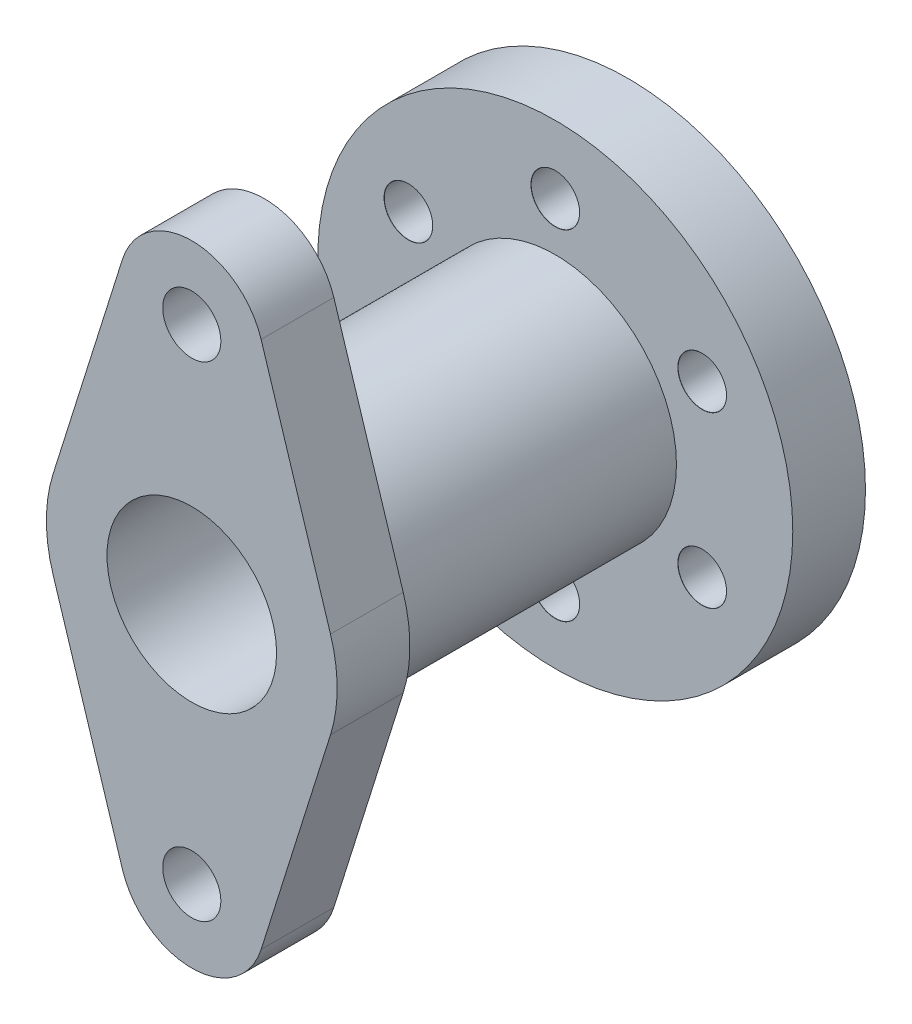
ISO-10303-21;
HEADER;
FILE_DESCRIPTION(('STEP AP214'),'2;1');
FILE_NAME('part.step','',(''),(''),'','','');
FILE_SCHEMA(('AUTOMOTIVE_DESIGN { 1 0 10303 214 1 1 1 1 }'));
ENDSEC;
DATA;
#1=APPLICATION_CONTEXT('core data for automotive mechanical design processes');
#2=APPLICATION_PROTOCOL_DEFINITION('international standard','automotive_design',2000,#1);
#3=PRODUCT_CONTEXT('',#1,'mechanical');
#4=PRODUCT('Part','Part','',(#3));
#5=PRODUCT_RELATED_PRODUCT_CATEGORY('part','',(#4));
#6=PRODUCT_DEFINITION_FORMATION('','',#4);
#7=PRODUCT_DEFINITION_CONTEXT('part definition',#1,'design');
#8=PRODUCT_DEFINITION('design','',#6,#7);
#9=PRODUCT_DEFINITION_SHAPE('','',#8);
#10=(LENGTH_UNIT() NAMED_UNIT(*) SI_UNIT(.MILLI.,.METRE.));
#11=(NAMED_UNIT(*) PLANE_ANGLE_UNIT() SI_UNIT($,.RADIAN.));
#12=(NAMED_UNIT(*) SI_UNIT($,.STERADIAN.) SOLID_ANGLE_UNIT());
#13=UNCERTAINTY_MEASURE_WITH_UNIT(LENGTH_MEASURE(1.E-05),#10,'distance_accuracy_value','');
#14=(GEOMETRIC_REPRESENTATION_CONTEXT(3) GLOBAL_UNCERTAINTY_ASSIGNED_CONTEXT((#13)) GLOBAL_UNIT_ASSIGNED_CONTEXT((#10,
#11,#12)) REPRESENTATION_CONTEXT('',''));
#15=CARTESIAN_POINT('',(0.,0.,0.));
#16=DIRECTION('',(0.,0.,1.));
#17=DIRECTION('',(1.,0.,0.));
#18=AXIS2_PLACEMENT_3D('',#15,#16,#17);
#19=CARTESIAN_POINT('',(0.,0.,90.));
#20=DIRECTION('',(0.,0.,-1.));
#21=DIRECTION('',(-1.,0.,0.));
#22=AXIS2_PLACEMENT_3D('',#19,#20,#21);
#23=CYLINDRICAL_SURFACE('',#22,13.);
#24=CARTESIAN_POINT('',(0.,0.,0.));
#25=DIRECTION('',(0.,0.,1.));
#26=DIRECTION('',(1.,0.,0.));
#27=AXIS2_PLACEMENT_3D('',#24,#25,#26);
#28=CIRCLE('',#27,13.);
#29=CARTESIAN_POINT('',(-13.,0.,0.));
#30=VERTEX_POINT('',#29);
#31=EDGE_CURVE('E179',#30,#30,#28,.T.);
#32=CARTESIAN_POINT('',(0.,0.,60.));
#33=DIRECTION('',(0.,0.,1.));
#34=DIRECTION('',(1.,0.,0.));
#35=AXIS2_PLACEMENT_3D('',#32,#33,#34);
#36=CIRCLE('',#35,13.);
#37=CARTESIAN_POINT('',(-13.,0.,60.));
#38=VERTEX_POINT('',#37);
#39=EDGE_CURVE('E51',#38,#38,#36,.T.);
#40=CARTESIAN_POINT('',(-13.,0.,0.));
#41=CARTESIAN_POINT('',(-13.,0.,0.624999999999988));
#42=CARTESIAN_POINT('',(-13.,0.,1.24999999999999));
#43=CARTESIAN_POINT('',(-13.,0.,2.49999999999999));
#44=CARTESIAN_POINT('',(-13.,0.,3.12499999999999));
#45=CARTESIAN_POINT('',(-13.,0.,4.37499999999999));
#46=CARTESIAN_POINT('',(-13.,0.,4.99999999999999));
#47=CARTESIAN_POINT('',(-13.,0.,6.24999999999999));
#48=CARTESIAN_POINT('',(-13.,0.,6.87499999999999));
#49=CARTESIAN_POINT('',(-13.,0.,8.12499999999999));
#50=CARTESIAN_POINT('',(-13.,0.,8.74999999999999));
#51=CARTESIAN_POINT('',(-13.,0.,9.99999999999999));
#52=CARTESIAN_POINT('',(-13.,0.,10.625));
#53=CARTESIAN_POINT('',(-13.,0.,11.875));
#54=CARTESIAN_POINT('',(-13.,0.,12.5));
#55=CARTESIAN_POINT('',(-13.,0.,13.75));
#56=CARTESIAN_POINT('',(-13.,0.,14.375));
#57=CARTESIAN_POINT('',(-13.,0.,15.625));
#58=CARTESIAN_POINT('',(-13.,0.,16.25));
#59=CARTESIAN_POINT('',(-13.,0.,17.5));
#60=CARTESIAN_POINT('',(-13.,0.,18.125));
#61=CARTESIAN_POINT('',(-13.,0.,19.375));
#62=CARTESIAN_POINT('',(-13.,0.,20.));
#63=CARTESIAN_POINT('',(-13.,0.,21.25));
#64=CARTESIAN_POINT('',(-13.,0.,21.875));
#65=CARTESIAN_POINT('',(-13.,0.,23.125));
#66=CARTESIAN_POINT('',(-13.,0.,23.75));
#67=CARTESIAN_POINT('',(-13.,0.,25.));
#68=CARTESIAN_POINT('',(-13.,0.,25.625));
#69=CARTESIAN_POINT('',(-13.,0.,26.875));
#70=CARTESIAN_POINT('',(-13.,0.,27.5));
#71=CARTESIAN_POINT('',(-13.,0.,28.75));
#72=CARTESIAN_POINT('',(-13.,0.,29.375));
#73=CARTESIAN_POINT('',(-13.,0.,30.625));
#74=CARTESIAN_POINT('',(-13.,0.,31.25));
#75=CARTESIAN_POINT('',(-13.,0.,32.5));
#76=CARTESIAN_POINT('',(-13.,0.,33.125));
#77=CARTESIAN_POINT('',(-13.,0.,34.375));
#78=CARTESIAN_POINT('',(-13.,0.,35.));
#79=CARTESIAN_POINT('',(-13.,0.,36.25));
#80=CARTESIAN_POINT('',(-13.,0.,36.875));
#81=CARTESIAN_POINT('',(-13.,0.,38.125));
#82=CARTESIAN_POINT('',(-13.,0.,38.75));
#83=CARTESIAN_POINT('',(-13.,0.,40.));
#84=CARTESIAN_POINT('',(-13.,0.,40.625));
#85=CARTESIAN_POINT('',(-13.,0.,41.875));
#86=CARTESIAN_POINT('',(-13.,0.,42.5));
#87=CARTESIAN_POINT('',(-13.,0.,43.75));
#88=CARTESIAN_POINT('',(-13.,0.,44.375));
#89=CARTESIAN_POINT('',(-13.,0.,45.625));
#90=CARTESIAN_POINT('',(-13.,0.,46.25));
#91=CARTESIAN_POINT('',(-13.,0.,47.5));
#92=CARTESIAN_POINT('',(-13.,0.,48.125));
#93=CARTESIAN_POINT('',(-13.,0.,49.375));
#94=CARTESIAN_POINT('',(-13.,0.,50.));
#95=CARTESIAN_POINT('',(-13.,0.,51.25));
#96=CARTESIAN_POINT('',(-13.,0.,51.875));
#97=CARTESIAN_POINT('',(-13.,0.,53.125));
#98=CARTESIAN_POINT('',(-13.,0.,53.75));
#99=CARTESIAN_POINT('',(-13.,0.,55.));
#100=CARTESIAN_POINT('',(-13.,0.,55.625));
#101=CARTESIAN_POINT('',(-13.,0.,56.875));
#102=CARTESIAN_POINT('',(-13.,0.,57.5));
#103=CARTESIAN_POINT('',(-13.,0.,58.75));
#104=CARTESIAN_POINT('',(-13.,0.,59.375));
#105=CARTESIAN_POINT('',(-13.,0.,60.));
#106=B_SPLINE_CURVE_WITH_KNOTS('',3,(#40,#41,#42,#43,#44,#45,#46,#47,#48,#49,#50,#51,#52,#53,
#54,#55,#56,#57,#58,#59,#60,#61,#62,#63,#64,#65,#66,#67,#68,#69,#70,#71,#72,#73,#74,#75,#76,#77,
#78,#79,#80,#81,#82,#83,#84,#85,#86,#87,#88,#89,#90,#91,#92,#93,#94,#95,#96,#97,#98,#99,#100,
#101,#102,#103,#104,#105),.UNSPECIFIED.,.F.,.F.,(4,2,2,2,2,2,2,2,2,2,2,2,2,2,2,2,2,2,2,2,2,2,2,
2,2,2,2,2,2,2,2,2,4),(0.,1.875,3.75,5.62500000000001,7.50000000000001,9.37500000000001,11.25,
13.125,15.,16.875,18.75,20.625,22.5,24.375,26.25,28.125,30.,31.875,33.75,35.625,37.5,39.375,
41.25,43.125,45.,46.875,48.75,50.625,52.5,54.375,56.25,58.125,60.),.UNSPECIFIED.);
#107=EDGE_CURVE('BSEAM50',#30,#38,#106,.T.);
#108=ORIENTED_EDGE('',*,*,#31,.F.);
#109=ORIENTED_EDGE('',*,*,#39,.T.);
#110=ORIENTED_EDGE('',*,*,#107,.T.);
#111=ORIENTED_EDGE('',*,*,#107,.F.);
#112=EDGE_LOOP('',(#108,#110,#109,#111));
#113=FACE_BOUND('',#112,.T.);
#114=ADVANCED_FACE('F50',(#113),#23,.F.);
#115=CARTESIAN_POINT('',(0.,0.,90.));
#116=DIRECTION('',(0.,0.,-1.));
#117=DIRECTION('',(-1.,0.,0.));
#118=AXIS2_PLACEMENT_3D('',#115,#116,#117);
#119=CYLINDRICAL_SURFACE('',#118,25.);
#120=CARTESIAN_POINT('',(0.,0.,15.));
#121=DIRECTION('',(0.,0.,1.));
#122=DIRECTION('',(1.,0.,0.));
#123=AXIS2_PLACEMENT_3D('',#120,#121,#122);
#124=CIRCLE('',#123,25.);
#125=CARTESIAN_POINT('',(-25.,0.,15.));
#126=VERTEX_POINT('',#125);
#127=EDGE_CURVE('E191',#126,#126,#124,.T.);
#128=CARTESIAN_POINT('',(0.,0.,75.));
#129=DIRECTION('',(0.,0.,1.));
#130=DIRECTION('',(1.,0.,0.));
#131=AXIS2_PLACEMENT_3D('',#128,#129,#130);
#132=CIRCLE('',#131,25.);
#133=CARTESIAN_POINT('',(-25.,0.,75.));
#134=VERTEX_POINT('',#133);
#135=EDGE_CURVE('E12',#134,#134,#132,.T.);
#136=CARTESIAN_POINT('',(-25.,0.,15.));
#137=CARTESIAN_POINT('',(-25.,0.,15.625));
#138=CARTESIAN_POINT('',(-25.,0.,16.25));
#139=CARTESIAN_POINT('',(-25.,0.,17.5));
#140=CARTESIAN_POINT('',(-25.,0.,18.125));
#141=CARTESIAN_POINT('',(-25.,0.,19.375));
#142=CARTESIAN_POINT('',(-25.,0.,20.));
#143=CARTESIAN_POINT('',(-25.,0.,21.25));
#144=CARTESIAN_POINT('',(-25.,0.,21.875));
#145=CARTESIAN_POINT('',(-25.,0.,23.125));
#146=CARTESIAN_POINT('',(-25.,0.,23.75));
#147=CARTESIAN_POINT('',(-25.,0.,25.));
#148=CARTESIAN_POINT('',(-25.,0.,25.625));
#149=CARTESIAN_POINT('',(-25.,0.,26.875));
#150=CARTESIAN_POINT('',(-25.,0.,27.5));
#151=CARTESIAN_POINT('',(-25.,0.,28.75));
#152=CARTESIAN_POINT('',(-25.,0.,29.375));
#153=CARTESIAN_POINT('',(-25.,0.,30.625));
#154=CARTESIAN_POINT('',(-25.,0.,31.25));
#155=CARTESIAN_POINT('',(-25.,0.,32.5));
#156=CARTESIAN_POINT('',(-25.,0.,33.125));
#157=CARTESIAN_POINT('',(-25.,0.,34.375));
#158=CARTESIAN_POINT('',(-25.,0.,35.));
#159=CARTESIAN_POINT('',(-25.,0.,36.25));
#160=CARTESIAN_POINT('',(-25.,0.,36.875));
#161=CARTESIAN_POINT('',(-25.,0.,38.125));
#162=CARTESIAN_POINT('',(-25.,0.,38.75));
#163=CARTESIAN_POINT('',(-25.,0.,40.));
#164=CARTESIAN_POINT('',(-25.,0.,40.625));
#165=CARTESIAN_POINT('',(-25.,0.,41.875));
#166=CARTESIAN_POINT('',(-25.,0.,42.5));
#167=CARTESIAN_POINT('',(-25.,0.,43.75));
#168=CARTESIAN_POINT('',(-25.,0.,44.375));
#169=CARTESIAN_POINT('',(-25.,0.,45.625));
#170=CARTESIAN_POINT('',(-25.,0.,46.25));
#171=CARTESIAN_POINT('',(-25.,0.,47.5));
#172=CARTESIAN_POINT('',(-25.,0.,48.125));
#173=CARTESIAN_POINT('',(-25.,0.,49.375));
#174=CARTESIAN_POINT('',(-25.,0.,50.));
#175=CARTESIAN_POINT('',(-25.,0.,51.25));
#176=CARTESIAN_POINT('',(-25.,0.,51.875));
#177=CARTESIAN_POINT('',(-25.,0.,53.125));
#178=CARTESIAN_POINT('',(-25.,0.,53.75));
#179=CARTESIAN_POINT('',(-25.,0.,55.));
#180=CARTESIAN_POINT('',(-25.,0.,55.625));
#181=CARTESIAN_POINT('',(-25.,0.,56.875));
#182=CARTESIAN_POINT('',(-25.,0.,57.5));
#183=CARTESIAN_POINT('',(-25.,0.,58.75));
#184=CARTESIAN_POINT('',(-25.,0.,59.375));
#185=CARTESIAN_POINT('',(-25.,0.,60.625));
#186=CARTESIAN_POINT('',(-25.,0.,61.25));
#187=CARTESIAN_POINT('',(-25.,0.,62.5));
#188=CARTESIAN_POINT('',(-25.,0.,63.125));
#189=CARTESIAN_POINT('',(-25.,0.,64.375));
#190=CARTESIAN_POINT('',(-25.,0.,65.));
#191=CARTESIAN_POINT('',(-25.,0.,66.25));
#192=CARTESIAN_POINT('',(-25.,0.,66.875));
#193=CARTESIAN_POINT('',(-25.,0.,68.125));
#194=CARTESIAN_POINT('',(-25.,0.,68.75));
#195=CARTESIAN_POINT('',(-25.,0.,70.));
#196=CARTESIAN_POINT('',(-25.,0.,70.625));
#197=CARTESIAN_POINT('',(-25.,0.,71.875));
#198=CARTESIAN_POINT('',(-25.,0.,72.5));
#199=CARTESIAN_POINT('',(-25.,0.,73.75));
#200=CARTESIAN_POINT('',(-25.,0.,74.375));
#201=CARTESIAN_POINT('',(-25.,0.,75.));
#202=B_SPLINE_CURVE_WITH_KNOTS('',3,(#136,#137,#138,#139,#140,#141,#142,#143,#144,#145,#146,
#147,#148,#149,#150,#151,#152,#153,#154,#155,#156,#157,#158,#159,#160,#161,#162,#163,#164,#165,
#166,#167,#168,#169,#170,#171,#172,#173,#174,#175,#176,#177,#178,#179,#180,#181,#182,#183,#184,
#185,#186,#187,#188,#189,#190,#191,#192,#193,#194,#195,#196,#197,#198,#199,#200,#201),
.UNSPECIFIED.,.F.,.F.,(4,2,2,2,2,2,2,2,2,2,2,2,2,2,2,2,2,2,2,2,2,2,2,2,2,2,2,2,2,2,2,2,4),(0.,
1.875,3.75,5.62500000000001,7.50000000000001,9.37499999999999,11.25,13.125,15.,16.875,18.75,
20.625,22.5,24.375,26.25,28.125,30.,31.875,33.75,35.625,37.5,39.375,41.25,43.125,45.,46.875,
48.75,50.625,52.5,54.375,56.25,58.125,60.),.UNSPECIFIED.);
#203=EDGE_CURVE('BSEAM209',#126,#134,#202,.T.);
#204=ORIENTED_EDGE('',*,*,#127,.T.);
#205=ORIENTED_EDGE('',*,*,#135,.F.);
#206=ORIENTED_EDGE('',*,*,#203,.T.);
#207=ORIENTED_EDGE('',*,*,#203,.F.);
#208=EDGE_LOOP('',(#204,#206,#205,#207));
#209=FACE_BOUND('',#208,.T.);
#210=ADVANCED_FACE('F209',(#209),#119,.T.);
#211=CARTESIAN_POINT('',(0.,0.,15.));
#212=DIRECTION('',(0.,0.,-1.));
#213=DIRECTION('',(-1.,0.,0.));
#214=AXIS2_PLACEMENT_3D('',#211,#212,#213);
#215=CYLINDRICAL_SURFACE('',#214,49.);
#216=CARTESIAN_POINT('',(0.,0.,15.));
#217=DIRECTION('',(0.,0.,1.));
#218=DIRECTION('',(1.,0.,0.));
#219=AXIS2_PLACEMENT_3D('',#216,#217,#218);
#220=CIRCLE('',#219,49.);
#221=CARTESIAN_POINT('',(49.,0.,15.));
#222=VERTEX_POINT('',#221);
#223=EDGE_CURVE('E60',#222,#222,#220,.T.);
#224=ORIENTED_EDGE('',*,*,#223,.F.);
#225=EDGE_LOOP('',(#224));
#226=FACE_BOUND('',#225,.T.);
#227=CARTESIAN_POINT('',(0.,0.,0.));
#228=DIRECTION('',(0.,0.,1.));
#229=DIRECTION('',(1.,0.,0.));
#230=AXIS2_PLACEMENT_3D('',#227,#228,#229);
#231=CIRCLE('',#230,49.);
#232=CARTESIAN_POINT('',(49.,0.,0.));
#233=VERTEX_POINT('',#232);
#234=EDGE_CURVE('E189',#233,#233,#231,.T.);
#235=ORIENTED_EDGE('',*,*,#234,.T.);
#236=EDGE_LOOP('',(#235));
#237=FACE_BOUND('',#236,.T.);
#238=ADVANCED_FACE('F47',(#226,#237),#215,.T.);
#239=CARTESIAN_POINT('',(0.,0.,15.));
#240=DIRECTION('',(0.,0.,1.));
#241=DIRECTION('',(1.,0.,0.));
#242=AXIS2_PLACEMENT_3D('',#239,#240,#241);
#243=PLANE('',#242);
#244=CARTESIAN_POINT('',(0.,35.,15.));
#245=DIRECTION('',(0.,0.,1.));
#246=DIRECTION('',(1.,0.,0.));
#247=AXIS2_PLACEMENT_3D('',#244,#245,#246);
#248=CIRCLE('',#247,5.025);
#249=CARTESIAN_POINT('',(5.025,35.,15.));
#250=VERTEX_POINT('',#249);
#251=EDGE_CURVE('E297',#250,#250,#248,.T.);
#252=ORIENTED_EDGE('',*,*,#251,.F.);
#253=EDGE_LOOP('',(#252));
#254=FACE_BOUND('',#253,.T.);
#255=CARTESIAN_POINT('',(30.3108891324554,17.4999999999999,15.));
#256=DIRECTION('',(0.,0.,1.));
#257=DIRECTION('',(1.,0.,0.));
#258=AXIS2_PLACEMENT_3D('',#255,#256,#257);
#259=CIRCLE('',#258,5.025);
#260=CARTESIAN_POINT('',(35.3358891324554,17.4999999999999,15.));
#261=VERTEX_POINT('',#260);
#262=EDGE_CURVE('E302',#261,#261,#259,.T.);
#263=ORIENTED_EDGE('',*,*,#262,.F.);
#264=EDGE_LOOP('',(#263));
#265=FACE_BOUND('',#264,.T.);
#266=CARTESIAN_POINT('',(30.3108891324553,-17.5000000000001,15.));
#267=DIRECTION('',(0.,0.,1.));
#268=DIRECTION('',(1.,0.,0.));
#269=AXIS2_PLACEMENT_3D('',#266,#267,#268);
#270=CIRCLE('',#269,5.025);
#271=CARTESIAN_POINT('',(35.3358891324553,-17.5000000000001,15.));
#272=VERTEX_POINT('',#271);
#273=EDGE_CURVE('E308',#272,#272,#270,.T.);
#274=ORIENTED_EDGE('',*,*,#273,.F.);
#275=EDGE_LOOP('',(#274));
#276=FACE_BOUND('',#275,.T.);
#277=CARTESIAN_POINT('',(-2.44403693719019E-13,-35.,15.));
#278=DIRECTION('',(0.,0.,1.));
#279=DIRECTION('',(1.,0.,0.));
#280=AXIS2_PLACEMENT_3D('',#277,#278,#279);
#281=CIRCLE('',#280,5.025);
#282=CARTESIAN_POINT('',(5.02499999999976,-35.,15.));
#283=VERTEX_POINT('',#282);
#284=EDGE_CURVE('E309',#283,#283,#281,.T.);
#285=ORIENTED_EDGE('',*,*,#284,.F.);
#286=EDGE_LOOP('',(#285));
#287=FACE_BOUND('',#286,.T.);
#288=CARTESIAN_POINT('',(-30.3108891324555,-17.4999999999997,15.));
#289=DIRECTION('',(0.,0.,1.));
#290=DIRECTION('',(1.,0.,0.));
#291=AXIS2_PLACEMENT_3D('',#288,#289,#290);
#292=CIRCLE('',#291,5.025);
#293=CARTESIAN_POINT('',(-25.2858891324555,-17.4999999999997,15.));
#294=VERTEX_POINT('',#293);
#295=EDGE_CURVE('E314',#294,#294,#292,.T.);
#296=ORIENTED_EDGE('',*,*,#295,.F.);
#297=EDGE_LOOP('',(#296));
#298=FACE_BOUND('',#297,.T.);
#299=CARTESIAN_POINT('',(-30.3108891324552,17.5000000000004,15.));
#300=DIRECTION('',(0.,0.,1.));
#301=DIRECTION('',(1.,0.,0.));
#302=AXIS2_PLACEMENT_3D('',#299,#300,#301);
#303=CIRCLE('',#302,5.025);
#304=CARTESIAN_POINT('',(-25.2858891324552,17.5000000000004,15.));
#305=VERTEX_POINT('',#304);
#306=EDGE_CURVE('E318',#305,#305,#303,.T.);
#307=ORIENTED_EDGE('',*,*,#306,.F.);
#308=EDGE_LOOP('',(#307));
#309=FACE_BOUND('',#308,.T.);
#310=ORIENTED_EDGE('',*,*,#127,.F.);
#311=EDGE_LOOP('',(#310));
#312=FACE_BOUND('',#311,.T.);
#313=ORIENTED_EDGE('',*,*,#223,.T.);
#314=EDGE_LOOP('',(#313));
#315=FACE_BOUND('',#314,.T.);
#316=ADVANCED_FACE('F204',(#254,#265,#276,#287,#298,#309,#312,#315),#243,.T.);
#317=CARTESIAN_POINT('',(0.,0.,0.));
#318=DIRECTION('',(0.,0.,1.));
#319=DIRECTION('',(1.,0.,0.));
#320=AXIS2_PLACEMENT_3D('',#317,#318,#319);
#321=PLANE('',#320);
#322=CARTESIAN_POINT('',(0.,35.,0.));
#323=DIRECTION('',(0.,0.,1.));
#324=DIRECTION('',(1.,0.,0.));
#325=AXIS2_PLACEMENT_3D('',#322,#323,#324);
#326=CIRCLE('',#325,5.);
#327=CARTESIAN_POINT('',(5.,35.,0.));
#328=VERTEX_POINT('',#327);
#329=EDGE_CURVE('E402',#328,#328,#326,.T.);
#330=ORIENTED_EDGE('',*,*,#329,.T.);
#331=EDGE_LOOP('',(#330));
#332=FACE_BOUND('',#331,.T.);
#333=CARTESIAN_POINT('',(30.3108891324554,17.4999999999999,0.));
#334=DIRECTION('',(0.,0.,1.));
#335=DIRECTION('',(1.,0.,0.));
#336=AXIS2_PLACEMENT_3D('',#333,#334,#335);
#337=CIRCLE('',#336,4.99999999999999);
#338=CARTESIAN_POINT('',(35.3108891324554,17.4999999999999,0.));
#339=VERTEX_POINT('',#338);
#340=EDGE_CURVE('E409',#339,#339,#337,.T.);
#341=ORIENTED_EDGE('',*,*,#340,.T.);
#342=EDGE_LOOP('',(#341));
#343=FACE_BOUND('',#342,.T.);
#344=CARTESIAN_POINT('',(30.3108891324553,-17.5000000000001,0.));
#345=DIRECTION('',(0.,0.,1.));
#346=DIRECTION('',(1.,0.,0.));
#347=AXIS2_PLACEMENT_3D('',#344,#345,#346);
#348=CIRCLE('',#347,5.);
#349=CARTESIAN_POINT('',(35.3108891324553,-17.5000000000001,0.));
#350=VERTEX_POINT('',#349);
#351=EDGE_CURVE('E417',#350,#350,#348,.T.);
#352=ORIENTED_EDGE('',*,*,#351,.T.);
#353=EDGE_LOOP('',(#352));
#354=FACE_BOUND('',#353,.T.);
#355=CARTESIAN_POINT('',(-2.44403693719019E-13,-35.,0.));
#356=DIRECTION('',(0.,0.,1.));
#357=DIRECTION('',(1.,0.,0.));
#358=AXIS2_PLACEMENT_3D('',#355,#356,#357);
#359=CIRCLE('',#358,5.);
#360=CARTESIAN_POINT('',(4.99999999999975,-35.,0.));
#361=VERTEX_POINT('',#360);
#362=EDGE_CURVE('E424',#361,#361,#359,.T.);
#363=ORIENTED_EDGE('',*,*,#362,.T.);
#364=EDGE_LOOP('',(#363));
#365=FACE_BOUND('',#364,.T.);
#366=CARTESIAN_POINT('',(-30.3108891324555,-17.4999999999997,0.));
#367=DIRECTION('',(0.,0.,1.));
#368=DIRECTION('',(1.,0.,0.));
#369=AXIS2_PLACEMENT_3D('',#366,#367,#368);
#370=CIRCLE('',#369,5.);
#371=CARTESIAN_POINT('',(-25.3108891324555,-17.4999999999997,0.));
#372=VERTEX_POINT('',#371);
#373=EDGE_CURVE('E431',#372,#372,#370,.T.);
#374=ORIENTED_EDGE('',*,*,#373,.T.);
#375=EDGE_LOOP('',(#374));
#376=FACE_BOUND('',#375,.T.);
#377=CARTESIAN_POINT('',(-30.3108891324552,17.5000000000004,0.));
#378=DIRECTION('',(0.,0.,1.));
#379=DIRECTION('',(1.,0.,0.));
#380=AXIS2_PLACEMENT_3D('',#377,#378,#379);
#381=CIRCLE('',#380,5.);
#382=CARTESIAN_POINT('',(-25.3108891324552,17.5000000000004,0.));
#383=VERTEX_POINT('',#382);
#384=EDGE_CURVE('E225',#383,#383,#381,.T.);
#385=ORIENTED_EDGE('',*,*,#384,.T.);
#386=EDGE_LOOP('',(#385));
#387=FACE_BOUND('',#386,.T.);
#388=ORIENTED_EDGE('',*,*,#234,.F.);
#389=EDGE_LOOP('',(#388));
#390=FACE_BOUND('',#389,.T.);
#391=ORIENTED_EDGE('',*,*,#31,.T.);
#392=EDGE_LOOP('',(#391));
#393=FACE_BOUND('',#392,.T.);
#394=ADVANCED_FACE('F199',(#332,#343,#354,#365,#376,#387,#390,#393),#321,.F.);
#395=CARTESIAN_POINT('',(0.,0.,90.));
#396=DIRECTION('',(0.,0.,1.));
#397=DIRECTION('',(1.,0.,0.));
#398=AXIS2_PLACEMENT_3D('',#395,#396,#397);
#399=PLANE('',#398);
#400=CARTESIAN_POINT('',(0.,0.,90.));
#401=DIRECTION('',(0.,0.,1.));
#402=DIRECTION('',(1.,0.,0.));
#403=AXIS2_PLACEMENT_3D('',#400,#401,#402);
#404=CIRCLE('',#403,17.5);
#405=CARTESIAN_POINT('',(17.5,0.,90.));
#406=VERTEX_POINT('',#405);
#407=EDGE_CURVE('E220',#406,#406,#404,.T.);
#408=ORIENTED_EDGE('',*,*,#407,.F.);
#409=EDGE_LOOP('',(#408));
#410=FACE_BOUND('',#409,.T.);
#411=CARTESIAN_POINT('',(0.,-50.,90.));
#412=DIRECTION('',(0.,0.,1.));
#413=DIRECTION('',(1.,0.,0.));
#414=AXIS2_PLACEMENT_3D('',#411,#412,#413);
#415=CIRCLE('',#414,6.);
#416=CARTESIAN_POINT('',(6.,-50.,90.));
#417=VERTEX_POINT('',#416);
#418=EDGE_CURVE('E147',#417,#417,#415,.F.);
#419=ORIENTED_EDGE('',*,*,#418,.T.);
#420=EDGE_LOOP('',(#419));
#421=FACE_BOUND('',#420,.T.);
#422=CARTESIAN_POINT('',(0.,50.,90.));
#423=DIRECTION('',(0.,0.,1.));
#424=DIRECTION('',(1.,0.,0.));
#425=AXIS2_PLACEMENT_3D('',#422,#423,#424);
#426=CIRCLE('',#425,6.);
#427=CARTESIAN_POINT('',(6.,50.,90.));
#428=VERTEX_POINT('',#427);
#429=EDGE_CURVE('E153',#428,#428,#426,.T.);
#430=ORIENTED_EDGE('',*,*,#429,.F.);
#431=EDGE_LOOP('',(#430));
#432=FACE_BOUND('',#431,.T.);
#433=DIRECTION('',(0.3,0.953939201416946,0.));
#434=VECTOR('',#433,1.);
#435=CARTESIAN_POINT('',(28.6181760425084,-9.,90.));
#436=LINE('',#435,#434);
#437=CARTESIAN_POINT('',(14.3090880212542,-54.5,90.));
#438=VERTEX_POINT('',#437);
#439=CARTESIAN_POINT('',(28.6181760425084,-9.,90.));
#440=VERTEX_POINT('',#439);
#441=EDGE_CURVE('E156',#438,#440,#436,.T.);
#442=ORIENTED_EDGE('',*,*,#441,.T.);
#443=CARTESIAN_POINT('',(0.,0.,90.));
#444=DIRECTION('',(0.,0.,1.));
#445=DIRECTION('',(1.,0.,0.));
#446=AXIS2_PLACEMENT_3D('',#443,#444,#445);
#447=CIRCLE('',#446,30.);
#448=CARTESIAN_POINT('',(28.6181760425084,9.,90.));
#449=VERTEX_POINT('',#448);
#450=EDGE_CURVE('E157',#440,#449,#447,.T.);
#451=ORIENTED_EDGE('',*,*,#450,.T.);
#452=DIRECTION('',(0.3,-0.953939201416946,0.));
#453=VECTOR('',#452,1.);
#454=CARTESIAN_POINT('',(28.6181760425084,9.,90.));
#455=LINE('',#454,#453);
#456=CARTESIAN_POINT('',(14.3090880212542,54.5,90.));
#457=VERTEX_POINT('',#456);
#458=EDGE_CURVE('E165',#457,#449,#455,.T.);
#459=ORIENTED_EDGE('',*,*,#458,.F.);
#460=CARTESIAN_POINT('',(0.,50.,90.));
#461=DIRECTION('',(0.,0.,1.));
#462=DIRECTION('',(1.,0.,0.));
#463=AXIS2_PLACEMENT_3D('',#460,#461,#462);
#464=CIRCLE('',#463,15.);
#465=CARTESIAN_POINT('',(-14.3090880212542,54.5,90.));
#466=VERTEX_POINT('',#465);
#467=EDGE_CURVE('E164',#457,#466,#464,.T.);
#468=ORIENTED_EDGE('',*,*,#467,.T.);
#469=DIRECTION('',(-0.3,-0.953939201416946,0.));
#470=VECTOR('',#469,1.);
#471=CARTESIAN_POINT('',(-28.6181760425084,9.,90.));
#472=LINE('',#471,#470);
#473=CARTESIAN_POINT('',(-28.6181760425084,9.,90.));
#474=VERTEX_POINT('',#473);
#475=EDGE_CURVE('E169',#466,#474,#472,.T.);
#476=ORIENTED_EDGE('',*,*,#475,.T.);
#477=CARTESIAN_POINT('',(0.,0.,90.));
#478=DIRECTION('',(0.,0.,1.));
#479=DIRECTION('',(1.,0.,0.));
#480=AXIS2_PLACEMENT_3D('',#477,#478,#479);
#481=CIRCLE('',#480,30.);
#482=CARTESIAN_POINT('',(-28.6181760425084,-9.,90.));
#483=VERTEX_POINT('',#482);
#484=EDGE_CURVE('E171',#474,#483,#481,.T.);
#485=ORIENTED_EDGE('',*,*,#484,.T.);
#486=DIRECTION('',(-0.3,0.953939201416946,0.));
#487=VECTOR('',#486,1.);
#488=CARTESIAN_POINT('',(-28.6181760425084,-9.,90.));
#489=LINE('',#488,#487);
#490=CARTESIAN_POINT('',(-14.3090880212542,-54.5,90.));
#491=VERTEX_POINT('',#490);
#492=EDGE_CURVE('E92',#491,#483,#489,.T.);
#493=ORIENTED_EDGE('',*,*,#492,.F.);
#494=CARTESIAN_POINT('',(0.,-50.,90.));
#495=DIRECTION('',(0.,0.,1.));
#496=DIRECTION('',(1.,0.,0.));
#497=AXIS2_PLACEMENT_3D('',#494,#495,#496);
#498=CIRCLE('',#497,15.);
#499=EDGE_CURVE('E173',#438,#491,#498,.F.);
#500=ORIENTED_EDGE('',*,*,#499,.F.);
#501=EDGE_LOOP('',(#442,#451,#459,#468,#476,#485,#493,#500));
#502=FACE_BOUND('',#501,.T.);
#503=ADVANCED_FACE('F201',(#410,#421,#432,#502),#399,.T.);
#504=CARTESIAN_POINT('',(28.6181760425084,-9.,75.));
#505=DIRECTION('',(0.953939201416946,-0.3,0.));
#506=DIRECTION('',(0.3,0.953939201416946,0.));
#507=AXIS2_PLACEMENT_3D('',#504,#505,#506);
#508=PLANE('',#507);
#509=ORIENTED_EDGE('',*,*,#441,.F.);
#510=DIRECTION('',(0.,0.,1.));
#511=VECTOR('',#510,1.);
#512=CARTESIAN_POINT('',(14.3090880212542,-54.5,75.));
#513=LINE('',#512,#511);
#514=CARTESIAN_POINT('',(14.3090880212542,-54.5,75.));
#515=VERTEX_POINT('',#514);
#516=EDGE_CURVE('E64',#515,#438,#513,.T.);
#517=ORIENTED_EDGE('',*,*,#516,.F.);
#518=DIRECTION('',(0.3,0.953939201416946,0.));
#519=VECTOR('',#518,1.);
#520=CARTESIAN_POINT('',(28.6181760425084,-9.,75.));
#521=LINE('',#520,#519);
#522=CARTESIAN_POINT('',(28.6181760425084,-9.,75.));
#523=VERTEX_POINT('',#522);
#524=EDGE_CURVE('E232',#515,#523,#521,.T.);
#525=ORIENTED_EDGE('',*,*,#524,.T.);
#526=DIRECTION('',(0.,0.,1.));
#527=VECTOR('',#526,1.);
#528=CARTESIAN_POINT('',(28.6181760425084,-9.,75.));
#529=LINE('',#528,#527);
#530=EDGE_CURVE('E106',#523,#440,#529,.T.);
#531=ORIENTED_EDGE('',*,*,#530,.T.);
#532=EDGE_LOOP('',(#509,#517,#525,#531));
#533=FACE_BOUND('',#532,.T.);
#534=ADVANCED_FACE('F253',(#533),#508,.T.);
#535=CARTESIAN_POINT('',(0.,-50.,75.));
#536=DIRECTION('',(0.,0.,1.));
#537=DIRECTION('',(1.,0.,0.));
#538=AXIS2_PLACEMENT_3D('',#535,#536,#537);
#539=CYLINDRICAL_SURFACE('',#538,15.);
#540=ORIENTED_EDGE('',*,*,#499,.T.);
#541=DIRECTION('',(0.,0.,1.));
#542=VECTOR('',#541,1.);
#543=CARTESIAN_POINT('',(-14.3090880212542,-54.5,75.));
#544=LINE('',#543,#542);
#545=CARTESIAN_POINT('',(-14.3090880212542,-54.5,75.));
#546=VERTEX_POINT('',#545);
#547=EDGE_CURVE('E138',#546,#491,#544,.T.);
#548=ORIENTED_EDGE('',*,*,#547,.F.);
#549=CARTESIAN_POINT('',(0.,-50.,75.));
#550=DIRECTION('',(0.,0.,1.));
#551=DIRECTION('',(1.,0.,0.));
#552=AXIS2_PLACEMENT_3D('',#549,#550,#551);
#553=CIRCLE('',#552,15.);
#554=EDGE_CURVE('E131',#515,#546,#553,.F.);
#555=ORIENTED_EDGE('',*,*,#554,.F.);
#556=ORIENTED_EDGE('',*,*,#516,.T.);
#557=EDGE_LOOP('',(#540,#548,#555,#556));
#558=FACE_BOUND('',#557,.T.);
#559=ADVANCED_FACE('F252',(#558),#539,.T.);
#560=CARTESIAN_POINT('',(-28.6181760425084,-9.,75.));
#561=DIRECTION('',(0.953939201416946,0.3,0.));
#562=DIRECTION('',(-0.3,0.953939201416946,0.));
#563=AXIS2_PLACEMENT_3D('',#560,#561,#562);
#564=PLANE('',#563);
#565=ORIENTED_EDGE('',*,*,#492,.T.);
#566=DIRECTION('',(0.,0.,1.));
#567=VECTOR('',#566,1.);
#568=CARTESIAN_POINT('',(-28.6181760425084,-9.,75.));
#569=LINE('',#568,#567);
#570=CARTESIAN_POINT('',(-28.6181760425084,-9.,75.));
#571=VERTEX_POINT('',#570);
#572=EDGE_CURVE('E134',#571,#483,#569,.T.);
#573=ORIENTED_EDGE('',*,*,#572,.F.);
#574=DIRECTION('',(-0.3,0.953939201416946,0.));
#575=VECTOR('',#574,1.);
#576=CARTESIAN_POINT('',(-28.6181760425084,-9.,75.));
#577=LINE('',#576,#575);
#578=EDGE_CURVE('E124',#546,#571,#577,.T.);
#579=ORIENTED_EDGE('',*,*,#578,.F.);
#580=ORIENTED_EDGE('',*,*,#547,.T.);
#581=EDGE_LOOP('',(#565,#573,#579,#580));
#582=FACE_BOUND('',#581,.T.);
#583=ADVANCED_FACE('F136',(#582),#564,.F.);
#584=CARTESIAN_POINT('',(0.,0.,75.));
#585=DIRECTION('',(0.,0.,1.));
#586=DIRECTION('',(1.,0.,0.));
#587=AXIS2_PLACEMENT_3D('',#584,#585,#586);
#588=CYLINDRICAL_SURFACE('',#587,30.);
#589=ORIENTED_EDGE('',*,*,#484,.F.);
#590=DIRECTION('',(0.,0.,1.));
#591=VECTOR('',#590,1.);
#592=CARTESIAN_POINT('',(-28.6181760425084,9.,75.));
#593=LINE('',#592,#591);
#594=CARTESIAN_POINT('',(-28.6181760425084,9.,75.));
#595=VERTEX_POINT('',#594);
#596=EDGE_CURVE('E140',#595,#474,#593,.T.);
#597=ORIENTED_EDGE('',*,*,#596,.F.);
#598=CARTESIAN_POINT('',(0.,0.,75.));
#599=DIRECTION('',(0.,0.,1.));
#600=DIRECTION('',(1.,0.,0.));
#601=AXIS2_PLACEMENT_3D('',#598,#599,#600);
#602=CIRCLE('',#601,30.);
#603=EDGE_CURVE('E129',#595,#571,#602,.T.);
#604=ORIENTED_EDGE('',*,*,#603,.T.);
#605=ORIENTED_EDGE('',*,*,#572,.T.);
#606=EDGE_LOOP('',(#589,#597,#604,#605));
#607=FACE_BOUND('',#606,.T.);
#608=ADVANCED_FACE('F142',(#607),#588,.T.);
#609=CARTESIAN_POINT('',(-28.6181760425084,9.,75.));
#610=DIRECTION('',(-0.953939201416946,0.3,0.));
#611=DIRECTION('',(-0.3,-0.953939201416946,0.));
#612=AXIS2_PLACEMENT_3D('',#609,#610,#611);
#613=PLANE('',#612);
#614=ORIENTED_EDGE('',*,*,#475,.F.);
#615=DIRECTION('',(0.,0.,1.));
#616=VECTOR('',#615,1.);
#617=CARTESIAN_POINT('',(-14.3090880212542,54.5,75.));
#618=LINE('',#617,#616);
#619=CARTESIAN_POINT('',(-14.3090880212542,54.5,75.));
#620=VERTEX_POINT('',#619);
#621=EDGE_CURVE('E182',#620,#466,#618,.T.);
#622=ORIENTED_EDGE('',*,*,#621,.F.);
#623=DIRECTION('',(-0.3,-0.953939201416946,0.));
#624=VECTOR('',#623,1.);
#625=CARTESIAN_POINT('',(-28.6181760425084,9.,75.));
#626=LINE('',#625,#624);
#627=EDGE_CURVE('E141',#620,#595,#626,.T.);
#628=ORIENTED_EDGE('',*,*,#627,.T.);
#629=ORIENTED_EDGE('',*,*,#596,.T.);
#630=EDGE_LOOP('',(#614,#622,#628,#629));
#631=FACE_BOUND('',#630,.T.);
#632=ADVANCED_FACE('F246',(#631),#613,.T.);
#633=CARTESIAN_POINT('',(0.,50.,75.));
#634=DIRECTION('',(0.,0.,1.));
#635=DIRECTION('',(1.,0.,0.));
#636=AXIS2_PLACEMENT_3D('',#633,#634,#635);
#637=CYLINDRICAL_SURFACE('',#636,15.);
#638=ORIENTED_EDGE('',*,*,#467,.F.);
#639=DIRECTION('',(0.,0.,1.));
#640=VECTOR('',#639,1.);
#641=CARTESIAN_POINT('',(14.3090880212542,54.5,75.));
#642=LINE('',#641,#640);
#643=CARTESIAN_POINT('',(14.3090880212542,54.5,75.));
#644=VERTEX_POINT('',#643);
#645=EDGE_CURVE('E181',#644,#457,#642,.T.);
#646=ORIENTED_EDGE('',*,*,#645,.F.);
#647=CARTESIAN_POINT('',(0.,50.,75.));
#648=DIRECTION('',(0.,0.,1.));
#649=DIRECTION('',(1.,0.,0.));
#650=AXIS2_PLACEMENT_3D('',#647,#648,#649);
#651=CIRCLE('',#650,15.);
#652=EDGE_CURVE('E144',#644,#620,#651,.T.);
#653=ORIENTED_EDGE('',*,*,#652,.T.);
#654=ORIENTED_EDGE('',*,*,#621,.T.);
#655=EDGE_LOOP('',(#638,#646,#653,#654));
#656=FACE_BOUND('',#655,.T.);
#657=ADVANCED_FACE('F241',(#656),#637,.T.);
#658=CARTESIAN_POINT('',(28.6181760425084,9.,75.));
#659=DIRECTION('',(-0.953939201416946,-0.3,0.));
#660=DIRECTION('',(0.3,-0.953939201416946,0.));
#661=AXIS2_PLACEMENT_3D('',#658,#659,#660);
#662=PLANE('',#661);
#663=ORIENTED_EDGE('',*,*,#458,.T.);
#664=DIRECTION('',(0.,0.,1.));
#665=VECTOR('',#664,1.);
#666=CARTESIAN_POINT('',(28.6181760425084,9.,75.));
#667=LINE('',#666,#665);
#668=CARTESIAN_POINT('',(28.6181760425084,9.,75.));
#669=VERTEX_POINT('',#668);
#670=EDGE_CURVE('E183',#669,#449,#667,.T.);
#671=ORIENTED_EDGE('',*,*,#670,.F.);
#672=DIRECTION('',(0.3,-0.953939201416946,0.));
#673=VECTOR('',#672,1.);
#674=CARTESIAN_POINT('',(28.6181760425084,9.,75.));
#675=LINE('',#674,#673);
#676=EDGE_CURVE('E237',#644,#669,#675,.T.);
#677=ORIENTED_EDGE('',*,*,#676,.F.);
#678=ORIENTED_EDGE('',*,*,#645,.T.);
#679=EDGE_LOOP('',(#663,#671,#677,#678));
#680=FACE_BOUND('',#679,.T.);
#681=ADVANCED_FACE('F248',(#680),#662,.F.);
#682=CARTESIAN_POINT('',(0.,50.,75.));
#683=DIRECTION('',(0.,0.,1.));
#684=DIRECTION('',(1.,0.,0.));
#685=AXIS2_PLACEMENT_3D('',#682,#683,#684);
#686=CYLINDRICAL_SURFACE('',#685,6.);
#687=CARTESIAN_POINT('',(0.,50.,75.));
#688=DIRECTION('',(0.,0.,1.));
#689=DIRECTION('',(1.,0.,0.));
#690=AXIS2_PLACEMENT_3D('',#687,#688,#689);
#691=CIRCLE('',#690,6.);
#692=CARTESIAN_POINT('',(6.,50.,75.));
#693=VERTEX_POINT('',#692);
#694=EDGE_CURVE('E228',#693,#693,#691,.T.);
#695=ORIENTED_EDGE('',*,*,#694,.F.);
#696=EDGE_LOOP('',(#695));
#697=FACE_BOUND('',#696,.T.);
#698=ORIENTED_EDGE('',*,*,#429,.T.);
#699=EDGE_LOOP('',(#698));
#700=FACE_BOUND('',#699,.T.);
#701=ADVANCED_FACE('F275',(#697,#700),#686,.F.);
#702=CARTESIAN_POINT('',(0.,-50.,75.));
#703=DIRECTION('',(0.,0.,1.));
#704=DIRECTION('',(1.,0.,0.));
#705=AXIS2_PLACEMENT_3D('',#702,#703,#704);
#706=CYLINDRICAL_SURFACE('',#705,6.);
#707=CARTESIAN_POINT('',(0.,-50.,75.));
#708=DIRECTION('',(0.,0.,1.));
#709=DIRECTION('',(1.,0.,0.));
#710=AXIS2_PLACEMENT_3D('',#707,#708,#709);
#711=CIRCLE('',#710,6.);
#712=CARTESIAN_POINT('',(6.,-50.,75.));
#713=VERTEX_POINT('',#712);
#714=EDGE_CURVE('E176',#713,#713,#711,.F.);
#715=ORIENTED_EDGE('',*,*,#714,.T.);
#716=EDGE_LOOP('',(#715));
#717=FACE_BOUND('',#716,.T.);
#718=ORIENTED_EDGE('',*,*,#418,.F.);
#719=EDGE_LOOP('',(#718));
#720=FACE_BOUND('',#719,.T.);
#721=ADVANCED_FACE('F273',(#717,#720),#706,.F.);
#722=CARTESIAN_POINT('',(0.,0.,75.));
#723=DIRECTION('',(0.,0.,1.));
#724=DIRECTION('',(1.,0.,0.));
#725=AXIS2_PLACEMENT_3D('',#722,#723,#724);
#726=CYLINDRICAL_SURFACE('',#725,30.);
#727=ORIENTED_EDGE('',*,*,#450,.F.);
#728=ORIENTED_EDGE('',*,*,#530,.F.);
#729=CARTESIAN_POINT('',(0.,0.,75.));
#730=DIRECTION('',(0.,0.,1.));
#731=DIRECTION('',(1.,0.,0.));
#732=AXIS2_PLACEMENT_3D('',#729,#730,#731);
#733=CIRCLE('',#732,30.);
#734=EDGE_CURVE('E233',#523,#669,#733,.T.);
#735=ORIENTED_EDGE('',*,*,#734,.T.);
#736=ORIENTED_EDGE('',*,*,#670,.T.);
#737=EDGE_LOOP('',(#727,#728,#735,#736));
#738=FACE_BOUND('',#737,.T.);
#739=ADVANCED_FACE('F250',(#738),#726,.T.);
#740=CARTESIAN_POINT('',(0.,0.,75.));
#741=DIRECTION('',(0.,0.,1.));
#742=DIRECTION('',(1.,0.,0.));
#743=AXIS2_PLACEMENT_3D('',#740,#741,#742);
#744=PLANE('',#743);
#745=ORIENTED_EDGE('',*,*,#714,.F.);
#746=EDGE_LOOP('',(#745));
#747=FACE_BOUND('',#746,.T.);
#748=ORIENTED_EDGE('',*,*,#694,.T.);
#749=EDGE_LOOP('',(#748));
#750=FACE_BOUND('',#749,.T.);
#751=ORIENTED_EDGE('',*,*,#135,.T.);
#752=EDGE_LOOP('',(#751));
#753=FACE_BOUND('',#752,.T.);
#754=ORIENTED_EDGE('',*,*,#524,.F.);
#755=ORIENTED_EDGE('',*,*,#554,.T.);
#756=ORIENTED_EDGE('',*,*,#578,.T.);
#757=ORIENTED_EDGE('',*,*,#603,.F.);
#758=ORIENTED_EDGE('',*,*,#627,.F.);
#759=ORIENTED_EDGE('',*,*,#652,.F.);
#760=ORIENTED_EDGE('',*,*,#676,.T.);
#761=ORIENTED_EDGE('',*,*,#734,.F.);
#762=EDGE_LOOP('',(#754,#755,#756,#757,#758,#759,#760,#761));
#763=FACE_BOUND('',#762,.T.);
#764=ADVANCED_FACE('F127',(#747,#750,#753,#763),#744,.F.);
#765=CARTESIAN_POINT('',(0.,0.,60.));
#766=DIRECTION('',(0.,0.,1.));
#767=DIRECTION('',(1.,0.,0.));
#768=AXIS2_PLACEMENT_3D('',#765,#766,#767);
#769=CYLINDRICAL_SURFACE('',#768,17.5);
#770=CARTESIAN_POINT('',(0.,0.,60.));
#771=DIRECTION('',(0.,0.,1.));
#772=DIRECTION('',(1.,0.,0.));
#773=AXIS2_PLACEMENT_3D('',#770,#771,#772);
#774=CIRCLE('',#773,17.5);
#775=CARTESIAN_POINT('',(17.5,0.,60.));
#776=VERTEX_POINT('',#775);
#777=EDGE_CURVE('E214',#776,#776,#774,.T.);
#778=ORIENTED_EDGE('',*,*,#777,.F.);
#779=EDGE_LOOP('',(#778));
#780=FACE_BOUND('',#779,.T.);
#781=ORIENTED_EDGE('',*,*,#407,.T.);
#782=EDGE_LOOP('',(#781));
#783=FACE_BOUND('',#782,.T.);
#784=ADVANCED_FACE('F326',(#780,#783),#769,.F.);
#785=CARTESIAN_POINT('',(0.,0.,60.));
#786=DIRECTION('',(0.,0.,1.));
#787=DIRECTION('',(1.,0.,0.));
#788=AXIS2_PLACEMENT_3D('',#785,#786,#787);
#789=PLANE('',#788);
#790=ORIENTED_EDGE('',*,*,#39,.F.);
#791=EDGE_LOOP('',(#790));
#792=FACE_BOUND('',#791,.T.);
#793=ORIENTED_EDGE('',*,*,#777,.T.);
#794=EDGE_LOOP('',(#793));
#795=FACE_BOUND('',#794,.T.);
#796=ADVANCED_FACE('F332',(#792,#795),#789,.T.);
#797=CARTESIAN_POINT('',(-30.3108891324552,17.5000000000004,15.));
#798=DIRECTION('',(0.,0.,1.));
#799=DIRECTION('',(1.,0.,0.));
#800=AXIS2_PLACEMENT_3D('',#797,#798,#799);
#801=CYLINDRICAL_SURFACE('',#800,5.);
#802=ORIENTED_EDGE('',*,*,#384,.F.);
#803=EDGE_LOOP('',(#802));
#804=FACE_BOUND('',#803,.T.);
#805=CARTESIAN_POINT('',(-30.3108891324552,17.5000000000004,14.975));
#806=DIRECTION('',(0.,0.,1.));
#807=DIRECTION('',(1.,0.,0.));
#808=AXIS2_PLACEMENT_3D('',#805,#806,#807);
#809=CIRCLE('',#808,5.);
#810=CARTESIAN_POINT('',(-25.3108891324552,17.5000000000004,14.975));
#811=VERTEX_POINT('',#810);
#812=EDGE_CURVE('E432',#811,#811,#809,.T.);
#813=ORIENTED_EDGE('',*,*,#812,.T.);
#814=EDGE_LOOP('',(#813));
#815=FACE_BOUND('',#814,.T.);
#816=ADVANCED_FACE('F343',(#804,#815),#801,.F.);
#817=CARTESIAN_POINT('',(-30.3108891324552,17.5000000000004,15.));
#818=DIRECTION('',(0.,0.,1.));
#819=DIRECTION('',(1.,0.,0.));
#820=AXIS2_PLACEMENT_3D('',#817,#818,#819);
#821=CONICAL_SURFACE('',#820,5.025,0.785398163397483);
#822=ORIENTED_EDGE('',*,*,#812,.F.);
#823=EDGE_LOOP('',(#822));
#824=FACE_BOUND('',#823,.T.);
#825=ORIENTED_EDGE('',*,*,#306,.T.);
#826=EDGE_LOOP('',(#825));
#827=FACE_BOUND('',#826,.T.);
#828=ADVANCED_FACE('F348',(#824,#827),#821,.F.);
#829=CARTESIAN_POINT('',(-30.3108891324555,-17.4999999999997,15.));
#830=DIRECTION('',(0.,0.,1.));
#831=DIRECTION('',(1.,0.,0.));
#832=AXIS2_PLACEMENT_3D('',#829,#830,#831);
#833=CYLINDRICAL_SURFACE('',#832,5.);
#834=ORIENTED_EDGE('',*,*,#373,.F.);
#835=EDGE_LOOP('',(#834));
#836=FACE_BOUND('',#835,.T.);
#837=CARTESIAN_POINT('',(-30.3108891324555,-17.4999999999997,14.975));
#838=DIRECTION('',(0.,0.,1.));
#839=DIRECTION('',(1.,0.,0.));
#840=AXIS2_PLACEMENT_3D('',#837,#838,#839);
#841=CIRCLE('',#840,5.);
#842=CARTESIAN_POINT('',(-25.3108891324555,-17.4999999999997,14.975));
#843=VERTEX_POINT('',#842);
#844=EDGE_CURVE('E428',#843,#843,#841,.T.);
#845=ORIENTED_EDGE('',*,*,#844,.T.);
#846=EDGE_LOOP('',(#845));
#847=FACE_BOUND('',#846,.T.);
#848=ADVANCED_FACE('F353',(#836,#847),#833,.F.);
#849=CARTESIAN_POINT('',(-30.3108891324555,-17.4999999999997,15.));
#850=DIRECTION('',(0.,0.,1.));
#851=DIRECTION('',(1.,0.,0.));
#852=AXIS2_PLACEMENT_3D('',#849,#850,#851);
#853=CONICAL_SURFACE('',#852,5.025,0.785398163397483);
#854=ORIENTED_EDGE('',*,*,#844,.F.);
#855=EDGE_LOOP('',(#854));
#856=FACE_BOUND('',#855,.T.);
#857=ORIENTED_EDGE('',*,*,#295,.T.);
#858=EDGE_LOOP('',(#857));
#859=FACE_BOUND('',#858,.T.);
#860=ADVANCED_FACE('F359',(#856,#859),#853,.F.);
#861=CARTESIAN_POINT('',(-2.44403693719019E-13,-35.,15.));
#862=DIRECTION('',(0.,0.,1.));
#863=DIRECTION('',(1.,0.,0.));
#864=AXIS2_PLACEMENT_3D('',#861,#862,#863);
#865=CYLINDRICAL_SURFACE('',#864,5.);
#866=ORIENTED_EDGE('',*,*,#362,.F.);
#867=EDGE_LOOP('',(#866));
#868=FACE_BOUND('',#867,.T.);
#869=CARTESIAN_POINT('',(-2.44403693719019E-13,-35.,14.975));
#870=DIRECTION('',(0.,0.,1.));
#871=DIRECTION('',(1.,0.,0.));
#872=AXIS2_PLACEMENT_3D('',#869,#870,#871);
#873=CIRCLE('',#872,5.);
#874=CARTESIAN_POINT('',(4.99999999999975,-35.,14.975));
#875=VERTEX_POINT('',#874);
#876=EDGE_CURVE('E423',#875,#875,#873,.T.);
#877=ORIENTED_EDGE('',*,*,#876,.T.);
#878=EDGE_LOOP('',(#877));
#879=FACE_BOUND('',#878,.T.);
#880=ADVANCED_FACE('F362',(#868,#879),#865,.F.);
#881=CARTESIAN_POINT('',(-2.44403693719019E-13,-35.,15.));
#882=DIRECTION('',(0.,0.,1.));
#883=DIRECTION('',(1.,0.,0.));
#884=AXIS2_PLACEMENT_3D('',#881,#882,#883);
#885=CONICAL_SURFACE('',#884,5.025,0.785398163397483);
#886=ORIENTED_EDGE('',*,*,#876,.F.);
#887=EDGE_LOOP('',(#886));
#888=FACE_BOUND('',#887,.T.);
#889=ORIENTED_EDGE('',*,*,#284,.T.);
#890=EDGE_LOOP('',(#889));
#891=FACE_BOUND('',#890,.T.);
#892=ADVANCED_FACE('F368',(#888,#891),#885,.F.);
#893=CARTESIAN_POINT('',(30.3108891324553,-17.5000000000001,15.));
#894=DIRECTION('',(0.,0.,1.));
#895=DIRECTION('',(1.,0.,0.));
#896=AXIS2_PLACEMENT_3D('',#893,#894,#895);
#897=CYLINDRICAL_SURFACE('',#896,5.);
#898=ORIENTED_EDGE('',*,*,#351,.F.);
#899=EDGE_LOOP('',(#898));
#900=FACE_BOUND('',#899,.T.);
#901=CARTESIAN_POINT('',(30.3108891324553,-17.5000000000001,14.975));
#902=DIRECTION('',(0.,0.,1.));
#903=DIRECTION('',(1.,0.,0.));
#904=AXIS2_PLACEMENT_3D('',#901,#902,#903);
#905=CIRCLE('',#904,5.);
#906=CARTESIAN_POINT('',(35.3108891324553,-17.5000000000001,14.975));
#907=VERTEX_POINT('',#906);
#908=EDGE_CURVE('E413',#907,#907,#905,.T.);
#909=ORIENTED_EDGE('',*,*,#908,.T.);
#910=EDGE_LOOP('',(#909));
#911=FACE_BOUND('',#910,.T.);
#912=ADVANCED_FACE('F367',(#900,#911),#897,.F.);
#913=CARTESIAN_POINT('',(30.3108891324553,-17.5000000000001,15.));
#914=DIRECTION('',(0.,0.,1.));
#915=DIRECTION('',(1.,0.,0.));
#916=AXIS2_PLACEMENT_3D('',#913,#914,#915);
#917=CONICAL_SURFACE('',#916,5.025,0.785398163397344);
#918=ORIENTED_EDGE('',*,*,#908,.F.);
#919=EDGE_LOOP('',(#918));
#920=FACE_BOUND('',#919,.T.);
#921=ORIENTED_EDGE('',*,*,#273,.T.);
#922=EDGE_LOOP('',(#921));
#923=FACE_BOUND('',#922,.T.);
#924=ADVANCED_FACE('F372',(#920,#923),#917,.F.);
#925=CARTESIAN_POINT('',(30.3108891324554,17.4999999999999,15.));
#926=DIRECTION('',(0.,0.,1.));
#927=DIRECTION('',(1.,0.,0.));
#928=AXIS2_PLACEMENT_3D('',#925,#926,#927);
#929=CYLINDRICAL_SURFACE('',#928,4.99999999999999);
#930=ORIENTED_EDGE('',*,*,#340,.F.);
#931=EDGE_LOOP('',(#930));
#932=FACE_BOUND('',#931,.T.);
#933=CARTESIAN_POINT('',(30.3108891324554,17.4999999999999,14.975));
#934=DIRECTION('',(0.,0.,1.));
#935=DIRECTION('',(1.,0.,0.));
#936=AXIS2_PLACEMENT_3D('',#933,#934,#935);
#937=CIRCLE('',#936,4.99999999999999);
#938=CARTESIAN_POINT('',(35.3108891324554,17.4999999999999,14.975));
#939=VERTEX_POINT('',#938);
#940=EDGE_CURVE('E410',#939,#939,#937,.T.);
#941=ORIENTED_EDGE('',*,*,#940,.T.);
#942=EDGE_LOOP('',(#941));
#943=FACE_BOUND('',#942,.T.);
#944=ADVANCED_FACE('F378',(#932,#943),#929,.F.);
#945=CARTESIAN_POINT('',(30.3108891324554,17.4999999999999,15.));
#946=DIRECTION('',(0.,0.,1.));
#947=DIRECTION('',(1.,0.,0.));
#948=AXIS2_PLACEMENT_3D('',#945,#946,#947);
#949=CONICAL_SURFACE('',#948,5.025,0.785398163397622);
#950=ORIENTED_EDGE('',*,*,#940,.F.);
#951=EDGE_LOOP('',(#950));
#952=FACE_BOUND('',#951,.T.);
#953=ORIENTED_EDGE('',*,*,#262,.T.);
#954=EDGE_LOOP('',(#953));
#955=FACE_BOUND('',#954,.T.);
#956=ADVANCED_FACE('F385',(#952,#955),#949,.F.);
#957=CARTESIAN_POINT('',(0.,35.,15.));
#958=DIRECTION('',(0.,0.,1.));
#959=DIRECTION('',(1.,0.,0.));
#960=AXIS2_PLACEMENT_3D('',#957,#958,#959);
#961=CYLINDRICAL_SURFACE('',#960,5.);
#962=ORIENTED_EDGE('',*,*,#329,.F.);
#963=EDGE_LOOP('',(#962));
#964=FACE_BOUND('',#963,.T.);
#965=CARTESIAN_POINT('',(0.,35.,14.975));
#966=DIRECTION('',(0.,0.,1.));
#967=DIRECTION('',(1.,0.,0.));
#968=AXIS2_PLACEMENT_3D('',#965,#966,#967);
#969=CIRCLE('',#968,5.);
#970=CARTESIAN_POINT('',(5.,35.,14.975));
#971=VERTEX_POINT('',#970);
#972=EDGE_CURVE('E398',#971,#971,#969,.T.);
#973=ORIENTED_EDGE('',*,*,#972,.T.);
#974=EDGE_LOOP('',(#973));
#975=FACE_BOUND('',#974,.T.);
#976=ADVANCED_FACE('F387',(#964,#975),#961,.F.);
#977=CARTESIAN_POINT('',(0.,35.,15.));
#978=DIRECTION('',(0.,0.,1.));
#979=DIRECTION('',(1.,0.,0.));
#980=AXIS2_PLACEMENT_3D('',#977,#978,#979);
#981=CONICAL_SURFACE('',#980,5.025,0.785398163397483);
#982=ORIENTED_EDGE('',*,*,#972,.F.);
#983=EDGE_LOOP('',(#982));
#984=FACE_BOUND('',#983,.T.);
#985=ORIENTED_EDGE('',*,*,#251,.T.);
#986=EDGE_LOOP('',(#985));
#987=FACE_BOUND('',#986,.T.);
#988=ADVANCED_FACE('F388',(#984,#987),#981,.F.);
#989=CLOSED_SHELL('',(#114,#210,#238,#316,#394,#503,#534,#559,#583,#608,#632,#657,#681,#701,
#721,#739,#764,#784,#796,#816,#828,#848,#860,#880,#892,#912,#924,#944,#956,#976,#988));
#990=MANIFOLD_SOLID_BREP('B2',#989);
#991=ADVANCED_BREP_SHAPE_REPRESENTATION('',(#18,#990),#14);
#992=SHAPE_DEFINITION_REPRESENTATION(#9,#991);
ENDSEC;
END-ISO-10303-21;
